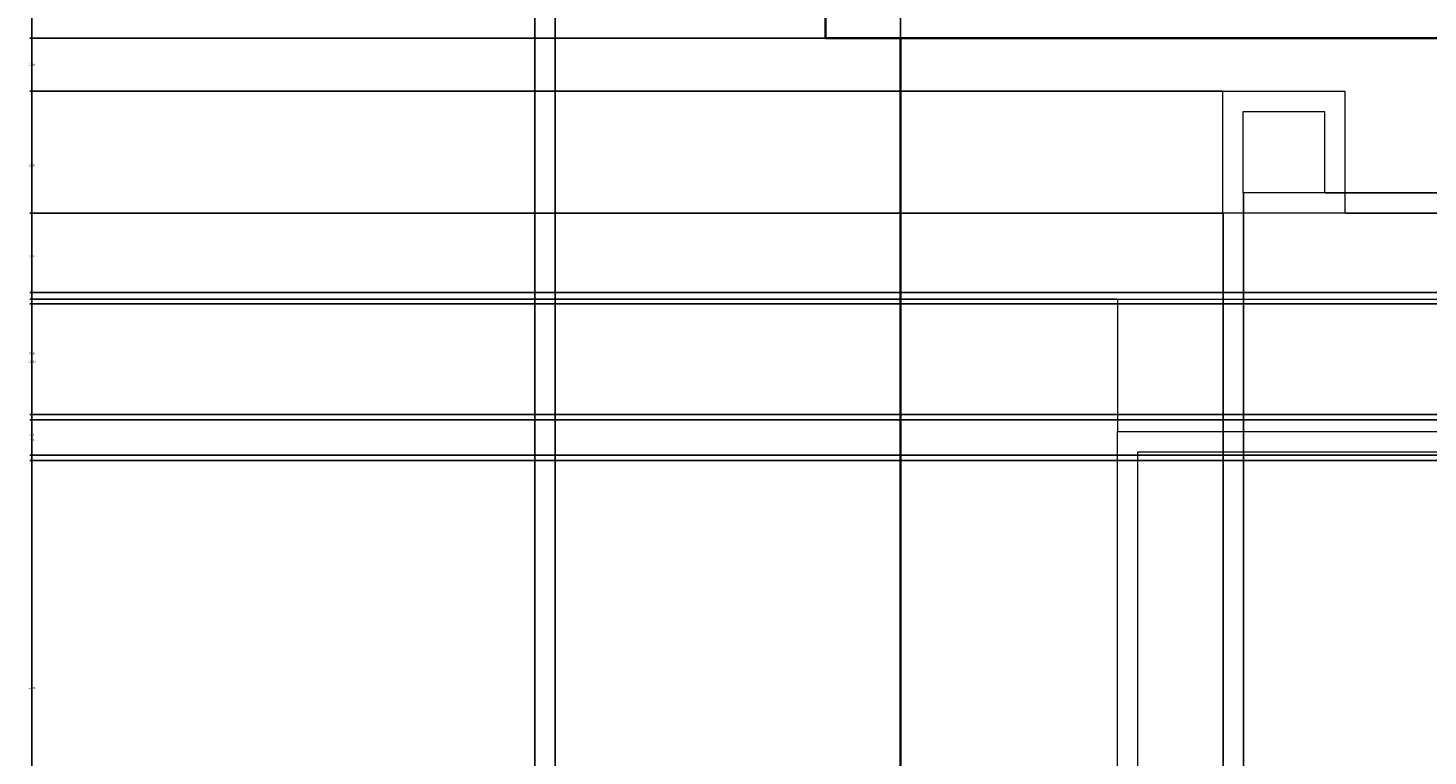
# Model space of a CAD drawing. Units: inches. Extents: x 1817 to 2378, y 1915 to 2370.
# Tile 2 of 8: x 1817 to 1955, y 2047 to 2119. Entities that reach past the tile are written whole.
import ezdxf

# ---------------------------------------------------------------- set-up
doc = ezdxf.new("R2010")
doc.units = ezdxf.units.IN
for name, color, linetype, lineweight in [('A-ANNO-DIMS', 2, 'Continuous', 18), ('A-ELEV', 7, 'Continuous', 35), ('A-GLAZ', 4, 'Continuous', 18)]:
    doc.layers.add(name, color=color, linetype=linetype, lineweight=lineweight)
doc.styles.get("Standard").update_dxf_attribs({"font": 'arial.ttf'})
doc.dimstyles.get("Standard").update_dxf_attribs({"dimtxt": 0.18, "dimasz": 0.18, "dimexe": 0.18, "dimexo": 0.0625, "dimgap": 0.09, "dimtad": 0, "dimtih": 1, "dimtoh": 1, "dimdec": 4, "dimzin": 0, "dimdsep": 46, "dimtxsty": 'Standard', "dimcen": 0.09, "dimadec": 0, "dimazin": 0, "dimtfac": 1, "dimtdec": 4, "dimtofl": 0, "dimtmove": 0, "dimatfit": 3, "dimfxl": 1, "dimtolj": 1, "dimtzin": 0, "dimarcsym": 0})

# ---------------------------------------------------------------- blocks, each defined once
blk = doc.blocks.new('WIN-SQ-900')
for points in [[(1924.43, 2204.58), (1960.43, 2204.58), (1960.43, 2217.58), (1924.43, 2217.58)], [(1924.43, 2204.58), (1960.43, 2204.58), (1960.43, 2168.58), (1924.43, 2168.58)], [(1926.43, 2202.58), (1958.43, 2202.58), (1958.43, 2170.58), (1926.43, 2170.58)]]:
    blk.add_lwpolyline(points, close=True)
blk = doc.blocks.new('VENT-300')
for points in [[(1936.66, 2237.16), (1948.66, 2237.16), (1948.66, 2225.16), (1936.66, 2225.16)], [(1938.66, 2235.16), (1946.66, 2235.16), (1946.66, 2227.16), (1938.66, 2227.16)]]:
    blk.add_lwpolyline(points, close=True)
blk = doc.blocks.new('*D10')
at = {"layer": 'A-ANNO-DIMS', "color": 0, "lineweight": -2, "transparency": 16777216}
for p, q in [((1867.08, 2019.57), (1867.08, 2369.94)), ((1867.26, 2369.76), (1884.87, 2369.76)), ((1902.9, 2369.76), (1885.3, 2369.76)), ((1903.08, 2019.57), (1903.08, 2369.94))]:
    blk.add_line(p, q, dxfattribs=at)
at = {"layer": 'A-ANNO-DIMS', "color": 0, "transparency": 16777216}
for points in [[(1867.26, 2369.79), (1867.26, 2369.73), (1867.08, 2369.76)], [(1902.9, 2369.79), (1902.9, 2369.73), (1903.08, 2369.76)]]:
    blk.add_solid(points, dxfattribs=at)
at = {"layer": 'Defpoints', "color": 0, "transparency": 16777216}
for p in [(1903.08, 2369.76), (1867.08, 2019.51), (1903.08, 2019.51)]:
    blk.add_point(p, dxfattribs=at)
at = {"layer": 'A-ANNO-DIMS', "color": 0, "transparency": 16777216, "insert": (1885.08, 2369.76), "char_height": 0.18, "attachment_point": 5}
blk.add_mtext('\\A1;36', dxfattribs=at)
blk = doc.blocks.new('*D13')
at = {"layer": 'A-ANNO-DIMS', "color": 0, "lineweight": -2, "transparency": 16777216}
for p, q in [((1934.83, 2100.21), (1934.83, 1915.08)), ((1924.43, 2042.72), (1924.43, 1915.08)), ((1924.61, 1915.26), (1929.31, 1915.26)), ((1934.65, 1915.26), (1929.94, 1915.26))]:
    blk.add_line(p, q, dxfattribs=at)
at = {"layer": 'A-ANNO-DIMS', "color": 0, "transparency": 16777216}
for points in [[(1924.61, 1915.29), (1924.61, 1915.23), (1924.43, 1915.26)], [(1934.65, 1915.29), (1934.65, 1915.23), (1934.83, 1915.26)]]:
    blk.add_solid(points, dxfattribs=at)
at = {"layer": 'Defpoints', "color": 0, "transparency": 16777216}
for p in [(1934.83, 2100.28), (1924.43, 2042.79), (1934.83, 1915.26)]:
    blk.add_point(p, dxfattribs=at)
at = {"layer": 'A-ANNO-DIMS', "color": 0, "transparency": 16777216, "insert": (1929.63, 1915.26), "char_height": 0.18, "attachment_point": 5}
blk.add_mtext('\\A1;10.4', dxfattribs=at)
blk = doc.blocks.new('*D14')
at = {"layer": 'A-ANNO-DIMS', "color": 0, "lineweight": -2, "transparency": 16777216}
for p, q in [((1934.83, 2100.21), (1934.83, 1915.08)), ((1960.43, 2042.72), (1960.43, 1915.08)), ((1935.01, 1915.26), (1947.3, 1915.26)), ((1960.25, 1915.26), (1947.95, 1915.26))]:
    blk.add_line(p, q, dxfattribs=at)
at = {"layer": 'A-ANNO-DIMS', "color": 0, "transparency": 16777216}
for points in [[(1935.01, 1915.29), (1935.01, 1915.23), (1934.83, 1915.26)], [(1960.25, 1915.29), (1960.25, 1915.23), (1960.43, 1915.26)]]:
    blk.add_solid(points, dxfattribs=at)
at = {"layer": 'Defpoints', "color": 0, "transparency": 16777216}
for p in [(1934.83, 2100.28), (1960.43, 2042.79), (1960.43, 1915.26)]:
    blk.add_point(p, dxfattribs=at)
at = {"layer": 'A-ANNO-DIMS', "color": 0, "transparency": 16777216, "insert": (1947.63, 1915.26), "char_height": 0.18, "attachment_point": 5}
blk.add_mtext('\\A1;25.6', dxfattribs=at)
blk = doc.blocks.new('*D23')
at = {"layer": 'A-ANNO-DIMS', "color": 0, "lineweight": -2, "transparency": 16777216}
for p, q in [((2320.11, 2156.45), (2320.11, 1915.08)), ((1867.08, 1965.45), (1867.08, 1915.08)), ((1867.26, 1915.26), (2093.3, 1915.26)), ((2319.93, 1915.26), (2093.89, 1915.26))]:
    blk.add_line(p, q, dxfattribs=at)
at = {"layer": 'A-ANNO-DIMS', "color": 0, "transparency": 16777216}
for points in [[(1867.26, 1915.29), (1867.26, 1915.23), (1867.08, 1915.26)], [(2319.93, 1915.29), (2319.93, 1915.23), (2320.11, 1915.26)]]:
    blk.add_solid(points, dxfattribs=at)
at = {"layer": 'Defpoints', "color": 0, "transparency": 16777216}
for p in [(2320.11, 2156.51), (1867.08, 1965.51), (2320.11, 1915.26)]:
    blk.add_point(p, dxfattribs=at)
at = {"layer": 'A-ANNO-DIMS', "color": 0, "transparency": 16777216, "insert": (2093.6, 1915.26), "char_height": 0.18, "attachment_point": 5}
blk.add_mtext('\\A1;453', dxfattribs=at)
blk = doc.blocks.new('*D54')
at = {"layer": 'A-ANNO-DIMS', "color": 0, "lineweight": -2, "transparency": 16777216}
for p, q in [((1901.02, 2343.51), (1817.4, 2343.51)), ((1817.58, 2343.33), (1817.58, 2154.69)), ((1817.58, 1965.69), (1817.58, 2154.33)), ((1867.02, 1965.51), (1817.4, 1965.51))]:
    blk.add_line(p, q, dxfattribs=at)
at = {"layer": 'A-ANNO-DIMS', "color": 0, "transparency": 16777216}
for points in [[(1817.55, 2343.33), (1817.61, 2343.33), (1817.58, 2343.51)], [(1817.55, 1965.69), (1817.61, 1965.69), (1817.58, 1965.51)]]:
    blk.add_solid(points, dxfattribs=at)
at = {"layer": 'Defpoints', "color": 0, "transparency": 16777216}
for p in [(1817.58, 2343.51), (1901.08, 2343.51), (1867.08, 1965.51)]:
    blk.add_point(p, dxfattribs=at)
at = {"layer": 'A-ANNO-DIMS', "color": 0, "transparency": 16777216, "insert": (1817.58, 2154.51), "char_height": 0.18, "attachment_point": 5}
blk.add_mtext('\\A1;378', dxfattribs=at)
blk = doc.blocks.new('*D58')
at = {"layer": 'A-ANNO-DIMS', "color": 0, "lineweight": -2, "transparency": 16777216}
for p, q in [((1934.76, 2100.28), (1817.4, 2100.28)), ((1817.58, 2100.1), (1817.58, 2096.21)), ((1817.58, 2091.97), (1817.58, 2095.85)), ((1924.36, 2091.79), (1817.4, 2091.79))]:
    blk.add_line(p, q, dxfattribs=at)
at = {"layer": 'A-ANNO-DIMS', "color": 0, "transparency": 16777216}
for points in [[(1817.55, 2100.1), (1817.61, 2100.1), (1817.58, 2100.28)], [(1817.55, 2091.97), (1817.61, 2091.97), (1817.58, 2091.79)]]:
    blk.add_solid(points, dxfattribs=at)
at = {"layer": 'Defpoints', "color": 0, "transparency": 16777216}
for p in [(1817.58, 2100.28), (1934.83, 2100.28), (1924.43, 2091.79)]:
    blk.add_point(p, dxfattribs=at)
at = {"layer": 'A-ANNO-DIMS', "color": 0, "transparency": 16777216, "insert": (1817.58, 2096.03), "char_height": 0.18, "attachment_point": 5}
blk.add_mtext('\\A1;8.49', dxfattribs=at)
blk = doc.blocks.new('*D59')
at = {"layer": 'A-ANNO-DIMS', "color": 0, "lineweight": -2, "transparency": 16777216}
for p, q in [((1903.02, 2117.51), (1817.4, 2117.51)), ((1817.58, 2117.33), (1817.58, 2115.07)), ((1817.58, 2112.46), (1817.58, 2114.71)), ((1934.76, 2112.28), (1817.4, 2112.28))]:
    blk.add_line(p, q, dxfattribs=at)
at = {"layer": 'A-ANNO-DIMS', "color": 0, "transparency": 16777216}
for points in [[(1817.55, 2117.33), (1817.61, 2117.33), (1817.58, 2117.51)], [(1817.55, 2112.46), (1817.61, 2112.46), (1817.58, 2112.28)]]:
    blk.add_solid(points, dxfattribs=at)
at = {"layer": 'Defpoints', "color": 0, "transparency": 16777216}
for p in [(1817.58, 2117.51), (1903.08, 2117.51), (1934.83, 2112.28)]:
    blk.add_point(p, dxfattribs=at)
at = {"layer": 'A-ANNO-DIMS', "color": 0, "transparency": 16777216, "insert": (1817.58, 2114.89), "char_height": 0.18, "attachment_point": 5}
blk.add_mtext('\\A1;5.233', dxfattribs=at)
blk = doc.blocks.new('*D60')
at = {"layer": 'A-ANNO-DIMS', "color": 0, "lineweight": -2, "transparency": 16777216}
for p, q in [((1903.02, 2127.51), (1817.4, 2127.51)), ((1817.58, 2127.33), (1817.58, 2122.69)), ((1817.58, 2117.69), (1817.58, 2122.33)), ((1895.63, 2117.51), (1817.4, 2117.51))]:
    blk.add_line(p, q, dxfattribs=at)
at = {"layer": 'A-ANNO-DIMS', "color": 0, "transparency": 16777216}
for points in [[(1817.55, 2127.33), (1817.61, 2127.33), (1817.58, 2127.51)], [(1817.55, 2117.69), (1817.61, 2117.69), (1817.58, 2117.51)]]:
    blk.add_solid(points, dxfattribs=at)
at = {"layer": 'Defpoints', "color": 0, "transparency": 16777216}
for p in [(1817.58, 2127.51), (1903.08, 2127.51), (1895.7, 2117.51)]:
    blk.add_point(p, dxfattribs=at)
at = {"layer": 'A-ANNO-DIMS', "color": 0, "transparency": 16777216, "insert": (1817.58, 2122.51), "char_height": 0.18, "attachment_point": 5}
blk.add_mtext('\\A1;10', dxfattribs=at)
blk = doc.blocks.new('*D81')
at = {"layer": 'A-ANNO-DIMS', "color": 0, "lineweight": -2, "transparency": 16777216}
for p, q in [((2198.53, 2117.51), (1817.4, 2117.51)), ((1817.58, 2117.33), (1817.58, 2105.16)), ((1817.58, 2092.63), (1817.58, 2104.8)), ((2123.56, 2092.45), (1817.4, 2092.45))]:
    blk.add_line(p, q, dxfattribs=at)
at = {"layer": 'A-ANNO-DIMS', "color": 0, "transparency": 16777216}
for points in [[(1817.55, 2117.33), (1817.61, 2117.33), (1817.58, 2117.51)], [(1817.55, 2092.63), (1817.61, 2092.63), (1817.58, 2092.45)]]:
    blk.add_solid(points, dxfattribs=at)
at = {"layer": 'Defpoints', "color": 0, "transparency": 16777216}
for p in [(1817.58, 2117.51), (2198.59, 2117.51), (2123.62, 2092.45)]:
    blk.add_point(p, dxfattribs=at)
at = {"layer": 'A-ANNO-DIMS', "color": 0, "transparency": 16777216, "insert": (1817.58, 2104.98), "char_height": 0.18, "attachment_point": 5}
blk.add_mtext('\\A1;25.06', dxfattribs=at)
blk = doc.blocks.new('*D83')
at = {"layer": 'A-ANNO-DIMS', "color": 0, "lineweight": -2, "transparency": 16777216}
for p, q in [((1936.83, 2102.21), (1936.83, 1915.08)), ((1934.83, 2100.21), (1934.83, 1915.08)), ((1935.01, 1915.26), (1935.68, 1915.26)), ((1936.65, 1915.26), (1935.98, 1915.26))]:
    blk.add_line(p, q, dxfattribs=at)
at = {"layer": 'A-ANNO-DIMS', "color": 0, "transparency": 16777216}
for points in [[(1935.01, 1915.29), (1935.01, 1915.23), (1934.83, 1915.26)], [(1936.65, 1915.29), (1936.65, 1915.23), (1936.83, 1915.26)]]:
    blk.add_solid(points, dxfattribs=at)
at = {"layer": 'Defpoints', "color": 0, "transparency": 16777216}
for p in [(1936.83, 2102.28), (1934.83, 2100.28), (1936.83, 1915.26)]:
    blk.add_point(p, dxfattribs=at)
at = {"layer": 'A-ANNO-DIMS', "color": 0, "transparency": 16777216, "insert": (1935.83, 1915.26), "char_height": 0.18, "attachment_point": 5}
blk.add_mtext('\\A1;2', dxfattribs=at)
blk = doc.blocks.new('*D88')
at = {"layer": 'A-ANNO-DIMS', "color": 0, "lineweight": -2, "transparency": 16777216}
for p, q in [((1936.83, 2102.21), (1936.83, 1915.08)), ((1934.83, 2100.21), (1934.83, 1915.08)), ((1935.01, 1915.26), (1935.5, 1915.26)), ((1936.65, 1915.26), (1936.15, 1915.26))]:
    blk.add_line(p, q, dxfattribs=at)
at = {"layer": 'A-ANNO-DIMS', "color": 0, "transparency": 16777216}
for points in [[(1935.01, 1915.29), (1935.01, 1915.23), (1934.83, 1915.26)], [(1936.65, 1915.29), (1936.65, 1915.23), (1936.83, 1915.26)]]:
    blk.add_solid(points, dxfattribs=at)
at = {"layer": 'Defpoints', "color": 0, "transparency": 16777216}
for p in [(1936.83, 2102.28), (1934.83, 2100.28), (1936.83, 1915.26)]:
    blk.add_point(p, dxfattribs=at)
at = {"layer": 'A-ANNO-DIMS', "color": 0, "transparency": 16777216, "insert": (1935.83, 1915.26), "char_height": 0.18, "attachment_point": 5}
blk.add_mtext('\\A1;2.00', dxfattribs=at)
blk = doc.blocks.new('*D89')
at = {"layer": 'A-ANNO-DIMS', "color": 0, "lineweight": -2, "transparency": 16777216}
for p, q in [((1944.89, 2102.28), (2377.4, 2102.28)), ((2377.22, 2102.1), (2377.22, 2101.46)), ((1946.89, 2100.28), (2377.4, 2100.28)), ((2377.22, 2100.46), (2377.22, 2101.09))]:
    blk.add_line(p, q, dxfattribs=at)
at = {"layer": 'A-ANNO-DIMS', "color": 0, "transparency": 16777216}
for points in [[(2377.19, 2102.1), (2377.25, 2102.1), (2377.22, 2102.28)], [(2377.19, 2100.46), (2377.25, 2100.46), (2377.22, 2100.28)]]:
    blk.add_solid(points, dxfattribs=at)
at = {"layer": 'Defpoints', "color": 0, "transparency": 16777216}
for p in [(1944.83, 2102.28), (2377.22, 2102.28), (1946.83, 2100.28)]:
    blk.add_point(p, dxfattribs=at)
at = {"layer": 'A-ANNO-DIMS', "color": 0, "transparency": 16777216, "insert": (2377.22, 2101.28), "char_height": 0.18, "attachment_point": 5}
blk.add_mtext('\\A1;2.00', dxfattribs=at)
blk = doc.blocks.new('*D90')
at = {"layer": 'A-ANNO-DIMS', "color": 0, "lineweight": -2, "transparency": 16777216}
for p, q in [((2123.56, 2092.45), (1817.4, 2092.45)), ((1817.58, 2092.27), (1817.58, 2086.63)), ((1817.58, 2080.63), (1817.58, 2086.26)), ((2123.56, 2080.45), (1817.4, 2080.45))]:
    blk.add_line(p, q, dxfattribs=at)
at = {"layer": 'A-ANNO-DIMS', "color": 0, "transparency": 16777216}
for points in [[(1817.55, 2092.27), (1817.61, 2092.27), (1817.58, 2092.45)], [(1817.55, 2080.63), (1817.61, 2080.63), (1817.58, 2080.45)]]:
    blk.add_solid(points, dxfattribs=at)
at = {"layer": 'Defpoints', "color": 0, "transparency": 16777216}
for p in [(2123.62, 2092.45), (1817.58, 2080.45), (2123.62, 2080.45)]:
    blk.add_point(p, dxfattribs=at)
at = {"layer": 'A-ANNO-DIMS', "color": 0, "transparency": 16777216, "insert": (1817.58, 2086.45), "char_height": 0.18, "attachment_point": 5}
blk.add_mtext('\\A1;12.00', dxfattribs=at)
blk = doc.blocks.new('*D91')
at = {"layer": 'A-ANNO-DIMS', "color": 0, "lineweight": -2, "transparency": 16777216}
for p, q in [((2123.56, 2080.45), (1817.4, 2080.45)), ((1817.58, 2080.27), (1817.58, 2078.63)), ((1817.58, 2076.63), (1817.58, 2078.26)), ((2127.56, 2076.45), (1817.4, 2076.45))]:
    blk.add_line(p, q, dxfattribs=at)
at = {"layer": 'A-ANNO-DIMS', "color": 0, "transparency": 16777216}
for points in [[(1817.55, 2080.27), (1817.61, 2080.27), (1817.58, 2080.45)], [(1817.55, 2076.63), (1817.61, 2076.63), (1817.58, 2076.45)]]:
    blk.add_solid(points, dxfattribs=at)
at = {"layer": 'Defpoints', "color": 0, "transparency": 16777216}
for p in [(2123.62, 2080.45), (1817.58, 2076.45), (2127.62, 2076.45)]:
    blk.add_point(p, dxfattribs=at)
at = {"layer": 'A-ANNO-DIMS', "color": 0, "transparency": 16777216, "insert": (1817.58, 2078.45), "char_height": 0.18, "attachment_point": 5}
blk.add_mtext('\\A1;4.00', dxfattribs=at)
blk = doc.blocks.new('*D94')
at = {"layer": 'A-ANNO-DIMS', "color": 0, "lineweight": -2, "transparency": 16777216}
for p, q in [((2210.55, 2091.36), (1817.4, 2091.36)), ((1817.58, 2091.18), (1817.58, 2085.83)), ((1817.58, 2080.11), (1817.58, 2085.47)), ((2210.55, 2079.93), (1817.4, 2079.93))]:
    blk.add_line(p, q, dxfattribs=at)
at = {"layer": 'A-ANNO-DIMS', "color": 0, "transparency": 16777216}
for points in [[(1817.55, 2091.18), (1817.61, 2091.18), (1817.58, 2091.36)], [(1817.55, 2080.11), (1817.61, 2080.11), (1817.58, 2079.93)]]:
    blk.add_solid(points, dxfattribs=at)
at = {"layer": 'Defpoints', "color": 0, "transparency": 16777216}
for p in [(2210.62, 2091.36), (1817.58, 2079.93), (2210.62, 2079.93)]:
    blk.add_point(p, dxfattribs=at)
at = {"layer": 'A-ANNO-DIMS', "color": 0, "transparency": 16777216, "insert": (1817.58, 2085.65), "char_height": 0.18, "attachment_point": 5}
blk.add_mtext('\\A1;11.433', dxfattribs=at)
blk = doc.blocks.new('*D95')
at = {"layer": 'A-ANNO-DIMS', "color": 0, "lineweight": -2, "transparency": 16777216}
for p, q in [((2210.55, 2079.93), (1817.4, 2079.93)), ((1817.58, 2079.75), (1817.58, 2078.11)), ((1817.58, 2076.11), (1817.58, 2077.75)), ((2214.55, 2075.93), (1817.4, 2075.93))]:
    blk.add_line(p, q, dxfattribs=at)
at = {"layer": 'A-ANNO-DIMS', "color": 0, "transparency": 16777216}
for points in [[(1817.55, 2079.75), (1817.61, 2079.75), (1817.58, 2079.93)], [(1817.55, 2076.11), (1817.61, 2076.11), (1817.58, 2075.93)]]:
    blk.add_solid(points, dxfattribs=at)
at = {"layer": 'Defpoints', "color": 0, "transparency": 16777216}
for p in [(2210.62, 2079.93), (1817.58, 2075.93), (2214.62, 2075.93)]:
    blk.add_point(p, dxfattribs=at)
at = {"layer": 'A-ANNO-DIMS', "color": 0, "transparency": 16777216, "insert": (1817.58, 2077.93), "char_height": 0.18, "attachment_point": 5}
blk.add_mtext('\\A1;4.00', dxfattribs=at)
blk = doc.blocks.new('*D116')
at = {"layer": 'A-ANNO-DIMS', "color": 0, "lineweight": -2, "transparency": 16777216}
for p, q in [((1867.08, 2017.57), (1867.08, 2369.94)), ((1867.26, 2369.76), (1867.76, 2369.76)), ((1868.9, 2369.76), (1868.41, 2369.76)), ((1869.08, 2017.57), (1869.08, 2369.94))]:
    blk.add_line(p, q, dxfattribs=at)
at = {"layer": 'A-ANNO-DIMS', "color": 0, "transparency": 16777216}
for points in [[(1867.26, 2369.79), (1867.26, 2369.73), (1867.08, 2369.76)], [(1868.9, 2369.79), (1868.9, 2369.73), (1869.08, 2369.76)]]:
    blk.add_solid(points, dxfattribs=at)
at = {"layer": 'Defpoints', "color": 0, "transparency": 16777216}
for p in [(1869.08, 2369.76), (1867.08, 2017.51), (1869.08, 2017.51)]:
    blk.add_point(p, dxfattribs=at)
at = {"layer": 'A-ANNO-DIMS', "color": 0, "transparency": 16777216, "insert": (1868.08, 2369.76), "char_height": 0.18, "attachment_point": 5}
blk.add_mtext('\\A1;2.00', dxfattribs=at)
blk = doc.blocks.new('*D119')
at = {"layer": 'A-ANNO-DIMS', "color": 0, "lineweight": -2, "transparency": 16777216}
for p, q in [((1903.08, 1989.57), (1903.08, 2369.94)), ((1903.26, 2369.76), (2091.62, 2369.76)), ((2280.9, 2369.76), (2092.55, 2369.76)), ((2281.08, 1989.57), (2281.08, 2369.94))]:
    blk.add_line(p, q, dxfattribs=at)
at = {"layer": 'A-ANNO-DIMS', "color": 0, "transparency": 16777216}
for points in [[(1903.26, 2369.79), (1903.26, 2369.73), (1903.08, 2369.76)], [(2280.9, 2369.79), (2280.9, 2369.73), (2281.08, 2369.76)]]:
    blk.add_solid(points, dxfattribs=at)
at = {"layer": 'Defpoints', "color": 0, "transparency": 16777216}
for p in [(2281.08, 2369.76), (1903.08, 1989.51), (2281.08, 1989.51)]:
    blk.add_point(p, dxfattribs=at)
at = {"layer": 'A-ANNO-DIMS', "color": 0, "transparency": 16777216, "insert": (2092.08, 2369.76), "char_height": 0.18, "attachment_point": 5}
blk.add_mtext('\\A1;378.00', dxfattribs=at)
blk = doc.blocks.new('*D120')
at = {"layer": 'A-ANNO-DIMS', "color": 0, "lineweight": -2, "transparency": 16777216}
for p, q in [((1983.02, 2117.51), (1817.4, 2117.51)), ((1817.58, 2117.33), (1817.58, 2053.69)), ((1817.58, 1989.69), (1817.58, 2053.33)), ((1983.02, 1989.51), (1817.4, 1989.51))]:
    blk.add_line(p, q, dxfattribs=at)
at = {"layer": 'A-ANNO-DIMS', "color": 0, "transparency": 16777216}
for points in [[(1817.55, 2117.33), (1817.61, 2117.33), (1817.58, 2117.51)], [(1817.55, 1989.69), (1817.61, 1989.69), (1817.58, 1989.51)]]:
    blk.add_solid(points, dxfattribs=at)
at = {"layer": 'Defpoints', "color": 0, "transparency": 16777216}
for p in [(1817.58, 2117.51), (1983.08, 2117.51), (1983.08, 1989.51)]:
    blk.add_point(p, dxfattribs=at)
at = {"layer": 'A-ANNO-DIMS', "color": 0, "transparency": 16777216, "insert": (1817.58, 2053.51), "char_height": 0.18, "attachment_point": 5}
blk.add_mtext('\\A1;128.00', dxfattribs=at)

msp = doc.modelspace()

# ---------------------------------------------------------------- linework, layer by layer
at = {"layer": 'A-ELEV'}
for p, q in [((1895.6961, 2119.5087), (1895.6961, 2117.5087)), ((2198.5896, 2117.5087), (1895.6961, 2117.5087)), ((1903.0849, 1965.5087), (1903.0849, 2117.5087))]:
    msp.add_line(p, q, dxfattribs=at)

# ---------------------------------------------------------------- block references
at = {"layer": 'A-GLAZ'}
for name, p in [('VENT-300', (-1.8383, -124.8836)), ('WIN-SQ-900', (0, -125.7955))]:
    msp.add_blockref(name, p, dxfattribs=at)

# ---------------------------------------------------------------- dimensions: what is measured, and where the dimension line sits
at = {"layer": 'A-ANNO-DIMS'}
for base, p1, p2, override, picture, middle in [((1903.0849, 2369.7587), (1867.0849, 2019.5087), (1903.0849, 2019.5087), {"dimdec": 0, "dimlfac": 1, "dimrnd": 0, "dimzin": 0, "dimdsep": 46, "dimlunit": 2}, '*D10', (1885.0849, 2369.7587)), ((1869.0849, 2369.7587), (1867.0849, 2017.5087), (1869.0849, 2017.5087), {"dimdec": 2, "dimlfac": 1, "dimrnd": 0, "dimzin": 0, "dimdsep": 46, "dimlunit": 2}, '*D116', (1868.0849, 2369.7587)), ((2281.0849, 2369.7587), (1903.0849, 1989.5087), (2281.0849, 1989.5087), {"dimdec": 2, "dimlfac": 1, "dimrnd": 0, "dimzin": 0, "dimdsep": 46, "dimlunit": 2}, '*D119', (2092.0849, 2369.7587)), ((2320.1054, 1915.2587), (1867.0849, 1965.5087), (2320.1054, 2156.5133), {"dimdec": 0, "dimlfac": 1, "dimrnd": 0, "dimzin": 0, "dimdsep": 46, "dimlunit": 2}, '*D23', (2093.5951, 1915.2587)), ((1936.8265, 1915.2587), (1934.8265, 2100.2756), (1936.8265, 2102.2756), {"dimdec": 0, "dimlfac": 1, "dimrnd": 0, "dimzin": 0, "dimdsep": 46, "dimlunit": 2}, '*D83', (1935.8265, 1915.2587)), ((1936.8265, 1915.2587), (1934.8265, 2100.2756), (1936.8265, 2102.2756), {"dimdec": 2, "dimlfac": 1, "dimrnd": 0, "dimzin": 0, "dimdsep": 46, "dimlunit": 2}, '*D88', (1935.8265, 1915.2587)), ((1934.8265, 1915.2587), (1924.4258, 2042.7858), (1934.8265, 2100.2756), {"dimdec": 1, "dimlfac": 1, "dimrnd": 0, "dimzin": 0, "dimdsep": 46, "dimlunit": 2}, '*D13', (1929.6262, 1915.2587)), ((1960.4258, 1915.2587), (1934.8265, 2100.2756), (1960.4258, 2042.7858), {"dimdec": 1, "dimlfac": 1, "dimrnd": 0, "dimzin": 0, "dimdsep": 46, "dimlunit": 2}, '*D14', (1947.6262, 1915.2587))]:
    dim = msp.add_linear_dim(base=base, p1=p1, p2=p2, dimstyle='Standard', override=override, dxfattribs=at)
    dim.commit()
    dim.dimension.update_dxf_attribs({"geometry": picture, "text_midpoint": middle})
for base, p1, p2, override, picture, middle in [((1817.584, 2343.5087), (1867.0849, 1965.5087), (1901.0849, 2343.5087), {"dimdec": 0, "dimlfac": 1, "dimrnd": 0, "dimzin": 0, "dimdsep": 46, "dimlunit": 2}, '*D54', (1817.584, 2154.5087)), ((1817.584, 2127.5087), (1895.6961, 2117.5087), (1903.0849, 2127.5087), {"dimdec": 0, "dimlfac": 1, "dimrnd": 0, "dimzin": 0, "dimdsep": 46, "dimlunit": 2}, '*D60', (1817.584, 2122.5087)), ((1817.584, 2117.5087), (1983.0849, 1989.5087), (1983.0849, 2117.5087), {"dimdec": 2, "dimlfac": 1, "dimrnd": 0, "dimzin": 0, "dimdsep": 46, "dimlunit": 2}, '*D120', (1817.584, 2053.5087)), ((1817.584, 2117.5087), (1934.8265, 2112.2756), (1903.0849, 2117.5087), {"dimdec": 3, "dimlfac": 1, "dimrnd": 0, "dimzin": 0, "dimdsep": 46, "dimlunit": 2}, '*D59', (1817.584, 2114.8922)), ((1817.584, 2117.5087), (2123.6179, 2092.4468), (2198.5896, 2117.5087), {"dimdec": 2, "dimlfac": 1, "dimrnd": 0, "dimzin": 0, "dimdsep": 46, "dimlunit": 2}, '*D81', (1817.584, 2104.9777)), ((2377.2181, 2102.2756), (1946.8265, 2100.2756), (1944.8265, 2102.2756), {"dimdec": 2, "dimlfac": 1, "dimrnd": 0, "dimzin": 0, "dimdsep": 46, "dimlunit": 2}, '*D89', (2377.2181, 2101.2756)), ((1817.584, 2100.2756), (1924.4258, 2091.7858), (1934.8265, 2100.2756), {"dimdec": 2, "dimlfac": 1, "dimrnd": 0, "dimzin": 0, "dimdsep": 46, "dimlunit": 2}, '*D58', (1817.584, 2096.0307)), ((1817.584, 2080.4468), (2123.6179, 2092.4468), (2123.6179, 2080.4468), {"dimdec": 2, "dimlfac": 1, "dimrnd": 0, "dimzin": 0, "dimdsep": 46, "dimlunit": 2}, '*D90', (1817.584, 2086.4468)), ((1817.584, 2079.9313), (2210.6163, 2091.3647), (2210.6163, 2079.9313), {"dimdec": 3, "dimlfac": 1, "dimrnd": 0, "dimzin": 0, "dimdsep": 46, "dimlunit": 2}, '*D94', (1817.584, 2085.648)), ((1817.584, 2076.4468), (2123.6179, 2080.4468), (2127.6179, 2076.4468), {"dimdec": 2, "dimlfac": 1, "dimrnd": 0, "dimzin": 0, "dimdsep": 46, "dimlunit": 2}, '*D91', (1817.584, 2078.4468)), ((1817.584, 2075.9313), (2210.6163, 2079.9313), (2214.6163, 2075.9313), {"dimdec": 2, "dimlfac": 1, "dimrnd": 0, "dimzin": 0, "dimdsep": 46, "dimlunit": 2}, '*D95', (1817.584, 2077.9313))]:
    dim = msp.add_linear_dim(base=base, p1=p1, p2=p2, angle=90, dimstyle='Standard', override=override, dxfattribs=at)
    dim.commit()
    dim.dimension.update_dxf_attribs({"geometry": picture, "text_midpoint": middle})

doc.saveas('drawing.dxf')
